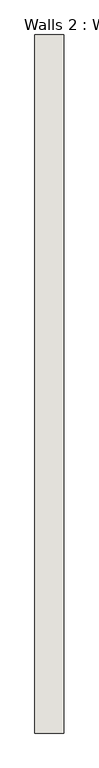
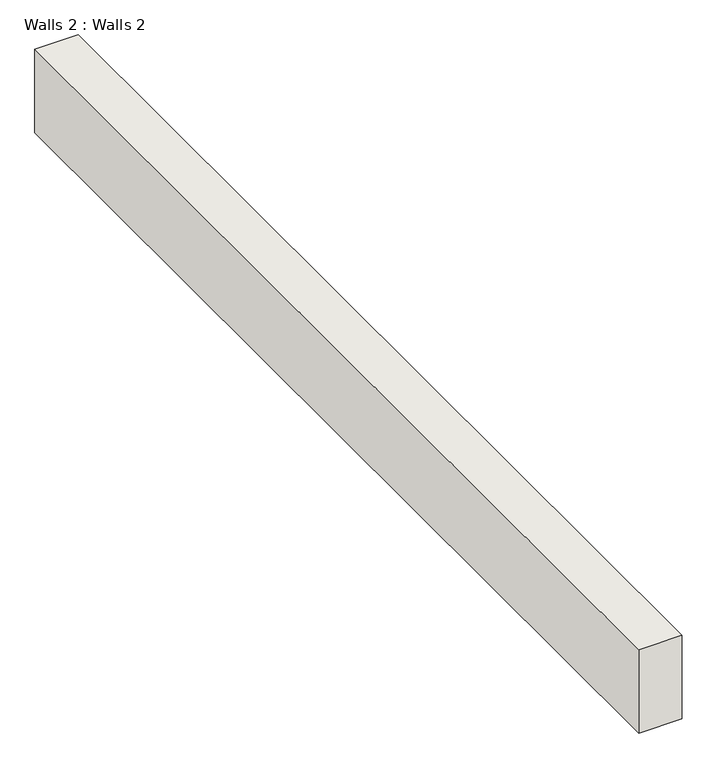
"""IFC4 building model written with IfcOpenShell, lengths in millimetres: wall geometry, Walls 2 : Walls 2."""

from ifc_helpers import new_model, si_unit, frame, origin, place, context, project, spatial, polyline, outline, extrude, source, transform, mapped, element, save


def walls_2_walls_2_334e7359(model_context):
    return source(origin(), model_context, "Body", "SweptSolid", [
        extrude(outline(polyline([(-2798.3625081, -8843.1874979), (-3129.5479903, -8843.1874979), (-3129.5479903, -798.6874979), (-2798.3625081, -798.6874979), (-2798.3625081, -8843.1874979)])), frame((0.0, 0.0, 2314.6286535), z_axis=(0.0, 0.0, 1.0), x_axis=(1.0, 0.0, 0.0)), (0.0, 0.0, 1.0), 678.7131983),
    ])


if __name__ == "__main__":
    model = new_model("IFC4")
    model_context = context("Model", 3, world=origin())
    ifc_project = project(units=[si_unit("LENGTHUNIT", "METRE", prefix="MILLI")], contexts=[model_context])
    site = spatial("IfcSite", under=ifc_project)
    building = spatial("IfcBuilding", under=site)
    placement = place(None, origin())
    walls_2_walls_2_shape = walls_2_walls_2_334e7359(model_context)
    element("IfcWall", 1, ObjectType="Walls 2 : Walls 2", at=placement, inside=building, context=model_context, shape_type="MappedRepresentation", body=[
        mapped(walls_2_walls_2_shape, transform((0.0, 0.0, 0.0), x_axis=(1.0, 0.0, 0.0), y_axis=(0.0, 1.0, 0.0), z_axis=(0.0, 0.0, 1.0))),
    ])
    save(model, "model.ifc")

# Revit data of these elements
# Element 1 (IfcWall, "Walls 2 : Walls 2")
#   Materials on its faces: "Default Wall"
# Materials
#   "Default Wall": colour RGB 80 80 80, transparency 0
